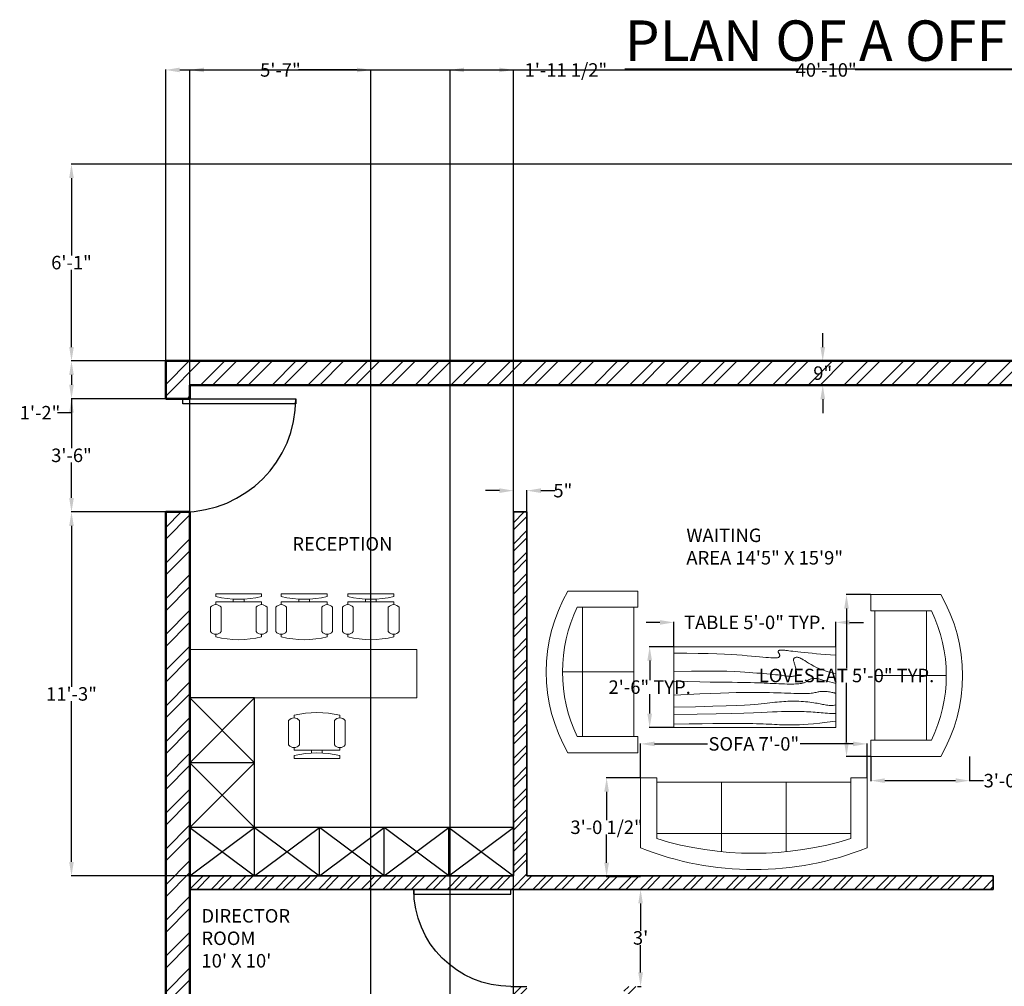
# Model space of a CAD drawing. Units: inches. Extents: x -355 to 263, y -871 to -163.
# Tile 5 of 6: x -355 to 10, y -521 to -163. Entities that reach past the tile are written whole.
import ezdxf

# ---------------------------------------------------------------- set-up
doc = ezdxf.new("R2010")
doc.units = ezdxf.units.IN
doc.header["$MEASUREMENT"] = 0
doc.layers.get('Defpoints').update_dxf_attribs({"color": 50})
for name, color, linetype, lineweight in [('A-ANNO-DIMS', 2, 'Continuous', 18), ('A-ANNO-TEXT', 7, 'Continuous', 25), ('A-AREA-IDEN', 7, 'Continuous', 18), ('A-FLOR-CASE', 9, 'Continuous', 25), ('A-WALL-PATT', 252, 'Continuous', 13)]:
    doc.layers.add(name, color=color, linetype=linetype, lineweight=lineweight)
for name, color, linetype, lineweight, plot in [('CHAIR', 8, 'Continuous', 18, False), ('DOOR', 4, 'Continuous', 25, False), ('IWAL', 7, 'Continuous', 35, False), ('OWALL', 7, 'Continuous', 50, False), ('SOFA', 8, 'Continuous', 18, False), ('TABLE', 8, 'Continuous', 18, False)]:
    doc.layers.add(name, color=color, linetype=linetype, lineweight=lineweight, plot=plot)
doc.styles.get("Standard").update_dxf_attribs({"font": 'arial.ttf'})
doc.dimstyles.get("Standard").update_dxf_attribs({"dimtxt": 5, "dimasz": 5.18, "dimexe": 0.18, "dimexo": 0.0625, "dimgap": 0.09, "dimtad": 0, "dimtih": 1, "dimtoh": 1, "dimdec": 0, "dimzin": 0, "dimdsep": 46, "dimlunit": 3, "dimtxsty": 'Standard', "dimcen": 0.09, "dimadec": 0, "dimazin": 0, "dimtfac": 1, "dimtdec": 0, "dimtofl": 0, "dimtmove": 0, "dimatfit": 3, "dimfxl": 1, "dimtolj": 1, "dimtzin": 0, "dimarcsym": 0})

# ---------------------------------------------------------------- blocks, each defined once
blk = doc.blocks.new('*U7')
for p, q in [((0, 0), (0, -6)), ((36, 0), (36, -6))]:
    blk.add_line(p, q)
blk.add_lwpolyline([(0, 0), (0, 36), (1.75, 36), (1.75, 0)], close=True)
blk.add_arc((0, 0), 36, 0, 90)
blk = doc.blocks.new('*U5')
for p, q in [((0, 0), (0, -6)), ((40, 0), (40, -6))]:
    blk.add_line(p, q)
blk.add_lwpolyline([(0, 0), (0, 40), (1.75, 40), (1.75, 0)], close=True)
blk.add_arc((0, 0), 40, 0, 90)
blk = doc.blocks.new('Chair - Desk')
for p, q in [((-8.5, 0), (-8.5, -1)), ((-8.5, 0), (8.5, 0)), ((8.5, 0), (8.5, -1)), ((-8.5, -3), (-8.5, -4)), ((-8.5, -3), (8.5, -3)), ((-2, -3), (-2, -1.9355)), ((2, -1.9576), (2, -3)), ((8.5, -3), (8.5, -4)), ((-10.5, -5), (-10.5, -14)), ((-6.5, -14), (-6.5, -5)), ((6.5, -5), (6.5, -14)), ((10.5, -14), (10.5, -5)), ((-8.5, -15), (-8.5, -16)), ((8.5, -15), (8.5, -16))]:
    blk.add_line(p, q)
for centre, radius, start, end in [((0, 34.625), 36.625, 256.5803, 283.4197), ((-8.5, -6.5), 2.5, 36.8699, 143.1301), ((8.5, -6.5), 2.5, 36.8699, 143.1301), ((-8.5, -12.5), 2.5, 216.8699, 323.1301), ((8.5, -12.5), 2.5, 216.8699, 323.1301), ((0, 19.625), 36.625, 256.5803, 283.4197)]:
    blk.add_arc(centre, radius, start, end)
blk = doc.blocks.new('Sofa - Roundback 7 ft.')
for p, q in [((-12.00002, -32.4421), (-12.00003, -6.5971)), ((11.99997, -32.4421), (11.99998, -6.5971)), ((-36.000027, -34), (-36.000027, -11.4696)), ((-35.999844, -13.3819), (35.9998, -13.3819)), ((35.99998, -34), (35.99998, -11.4696)), ((-36.000027, -32.4421), (35.99998, -32.4421))]:
    blk.add_line(p, q)
for points in [[(-36.000027, -34), (-42.000027, -34), (-42.000027, -8)], [(41.99998, -8), (41.99998, -34), (35.99998, -34)]]:
    blk.add_lwpolyline(points)
for centre, radius, start, end in [((0, -114.25), 114.25, 68.43141, 111.5686), ((-0.00001, -127.1968), 121.1968, 72.72033, 107.2797)]:
    blk.add_arc(centre, radius, start, end)
blk = doc.blocks.new('Sofa - Roundback Loveseat 5 ft.')
for p, q in [((0, -32.44198), (0, -5.99998)), ((-24, -33.99998), (-24, -11.46958)), ((-23.9998, -13.38178), (23.99986, -13.38178)), ((24.00004, -33.99998), (24.00004, -11.46958)), ((-24, -32.44198), (24.00004, -32.44198))]:
    blk.add_line(p, q)
for points in [[(-24, -33.99998), (-30, -33.99998), (-30, -7.99998)], [(30.00004, -7.99998), (30.00004, -33.99998), (24.00004, -33.99998)]]:
    blk.add_lwpolyline(points)
for centre, radius, start, end in [((0, -60.24998), 60.24998, 60.13715, 119.8628), ((0, -61.38438), 55.38444, 64.32083, 115.6792)]:
    blk.add_arc(centre, radius, start, end)
blk = doc.blocks.new('*D43')
at = {"layer": 'A-ANNO-DIMS', "color": 0, "lineweight": -2, "transparency": 16777216}
for p, q in [((-177.5, -337.37), (-182.68, -337.37)), ((-172.32, -345.22), (-172.32, -337.19)), ((-167.32, -345.22), (-167.32, -337.19)), ((-162.14, -337.37), (-156.96, -337.37))]:
    blk.add_line(p, q, dxfattribs=at)
at = {"layer": 'A-ANNO-DIMS', "color": 0, "lineweight": -3, "transparency": 16777216}
for points in [[(-177.5, -336.51), (-177.5, -338.24), (-172.32, -337.37)], [(-162.14, -336.51), (-162.14, -338.24), (-167.32, -337.37)]]:
    blk.add_solid(points, dxfattribs=at)
at = {"layer": 'Defpoints', "color": 0, "lineweight": -3, "transparency": 16777216}
for p in [(-167.32, -337.37), (-172.32, -345.28), (-167.32, -345.28)]:
    blk.add_point(p, dxfattribs=at)
at = {"layer": 'A-ANNO-DIMS', "color": 0, "transparency": 16777216, "insert": (-154, -337.37), "char_height": 5, "attachment_point": 5}
blk.add_mtext('\\A1;5"', dxfattribs=at)
blk = doc.blocks.new('*D44')
at = {"layer": 'A-ANNO-DIMS', "color": 0, "lineweight": -2, "transparency": 16777216}
for p, q in [((-57.59, -284.1), (-57.59, -278.92)), ((-80.81, -289.28), (-57.41, -289.28)), ((-80.81, -298.28), (-57.41, -298.28)), ((-57.59, -303.46), (-57.59, -308.64))]:
    blk.add_line(p, q, dxfattribs=at)
at = {"layer": 'A-ANNO-DIMS', "color": 0, "lineweight": -3, "transparency": 16777216}
for points in [[(-58.45, -284.1), (-56.72, -284.1), (-57.59, -289.28)], [(-58.45, -303.46), (-56.72, -303.46), (-57.59, -298.28)]]:
    blk.add_solid(points, dxfattribs=at)
at = {"layer": 'Defpoints', "color": 0, "lineweight": -3, "transparency": 16777216}
for p in [(-80.87, -289.28), (-80.87, -298.28), (-57.59, -298.28)]:
    blk.add_point(p, dxfattribs=at)
at = {"layer": 'A-ANNO-DIMS', "color": 0, "transparency": 16777216, "insert": (-57.59, -293.78), "char_height": 5, "attachment_point": 5}
blk.add_mtext('\\A1;9"', dxfattribs=at)
blk = doc.blocks.new('*D51')
at = {"layer": 'A-ANNO-DIMS', "color": 0, "lineweight": -2, "transparency": 16777216}
for p, q in [((-126.26, -485.28), (-124.98, -485.28)), ((-125.16, -490.46), (-125.16, -500.64)), ((-125.16, -516.1), (-125.16, -505.92)), ((-126.26, -521.28), (-124.98, -521.28))]:
    blk.add_line(p, q, dxfattribs=at)
at = {"layer": 'A-ANNO-DIMS', "color": 0, "lineweight": -3, "transparency": 16777216}
for points in [[(-126.02, -490.46), (-124.3, -490.46), (-125.16, -485.28)], [(-126.02, -516.1), (-124.3, -516.1), (-125.16, -521.28)]]:
    blk.add_solid(points, dxfattribs=at)
at = {"layer": 'Defpoints', "color": 0, "lineweight": -3, "transparency": 16777216}
for p in [(-126.32, -485.28), (-125.16, -485.28), (-126.32, -521.28)]:
    blk.add_point(p, dxfattribs=at)
at = {"layer": 'A-ANNO-DIMS', "color": 0, "transparency": 16777216, "insert": (-125.16, -503.28), "char_height": 5, "attachment_point": 5}
blk.add_mtext("\\A1;3'", dxfattribs=at)
blk = doc.blocks.new('Table - Rectangular Woodgrain 60 x 30 in.')
for p, q in [((0, 0), (0, -30)), ((60, 0), (0, 0)), ((60, -30), (60, 0)), ((0, -30), (60, -30))]:
    blk.add_line(p, q)
for points in [[(0, -2.4), (4.8155, -2.418), (9.0302, -2.4688), (12.709, -2.5477), (15.9167, -2.65), (18.7181, -2.7711), (21.1781, -2.9063), (23.3616, -3.0508), (25.3333, -3.2), (27.1477, -3.3495), (28.8172, -3.4958), (30.3437, -3.636), (31.7291, -3.7667), (32.9756, -3.8849), (34.0849, -3.9875), (35.059, -4.0714), (35.9, -4.1334), (36.6114, -4.1711), (37.2041, -4.1854), (37.6906, -4.1779), (38.0833, -4.15), (38.3948, -4.1034), (38.6375, -4.0396), (38.8239, -3.9602), (38.9666, -3.8667), (39.0764, -3.7608), (39.1573, -3.6448), (39.2116, -3.521), (39.2416, -3.3917), (39.2498, -3.2593), (39.2385, -3.1261), (39.21, -2.9944), (39.1666, -2.8667), (39.111, -2.7447), (39.0468, -2.6281), (38.978, -2.5163), (38.9083, -2.4083), (38.8418, -2.3035), (38.7823, -2.201), (38.7337, -2.1001), (38.7, -2), (38.6844, -1.9003), (38.6875, -1.8021), (38.7094, -1.707), (38.75, -1.6167), (38.8094, -1.5326), (38.8875, -1.4563), (38.9844, -1.3893), (39.1, -1.3333), (39.2351, -1.2896), (39.3937, -1.2583), (39.5804, -1.2396), (39.8, -1.2333), (40.057, -1.2396), (40.3562, -1.2583), (40.7023, -1.2896), (41.1, -1.3333), (41.5547, -1.3895), (42.0755, -1.4573), (42.6721, -1.5361), (43.3542, -1.625), (44.1316, -1.7233), (45.014, -1.8302), (46.0114, -1.9449), (47.1333, -2.0667), (48.3862, -2.1947), (49.7625, -2.3281), (51.2513, -2.4663), (52.8416, -2.6083), (54.5226, -2.7535), (56.2833, -2.9011), (58.1127, -3.0501), (60, -3.2)], [(0, -9.2), (6.5759, -9.0858), (11.9385, -9.0365), (16.2527, -9.0418), (19.6833, -9.0917), (22.3952, -9.1759), (24.5531, -9.2844), (26.322, -9.4069), (27.8666, -9.5333), (29.3241, -9.6553), (30.7203, -9.7719), (32.0532, -9.8837), (33.3208, -9.9917), (34.5213, -10.0965), (35.6526, -10.199), (36.7128, -10.2999), (37.7, -10.4), (38.6129, -10.4996), (39.4531, -10.5969), (40.223, -10.6895), (40.925, -10.775), (41.5613, -10.8512), (42.1344, -10.9156), (42.6465, -10.966), (43.1, -11), (43.4976, -11.0158), (43.8437, -11.0136), (44.143, -10.9942), (44.4, -10.9583), (44.6195, -10.9069), (44.8062, -10.8406), (44.9648, -10.7603), (45.1, -10.6667), (45.2155, -10.5598), (45.3114, -10.4365), (45.3871, -10.2929), (45.4416, -10.125), (45.4743, -9.929), (45.4844, -9.7011), (45.4709, -9.4371), (45.4333, -9.1333), (45.3716, -8.7883), (45.2896, -8.4104), (45.1919, -8.0107), (45.0833, -7.6), (44.9685, -7.1893), (44.8521, -6.7896), (44.7388, -6.4117), (44.6333, -6.0667), (44.54, -5.7628), (44.4614, -5.4979), (44.4001, -5.2675), (44.3583, -5.0667), (44.3384, -4.8909), (44.3427, -4.7354), (44.3736, -4.5956), (44.4333, -4.4667), (44.5236, -4.3453), (44.6427, -4.2333), (44.7884, -4.1339), (44.9583, -4.05), (45.1501, -3.9849), (45.3614, -3.9417), (45.59, -3.9234), (45.8333, -3.9333), (46.0915, -3.9749), (46.3734, -4.0531), (46.6906, -4.1736), (47.0542, -4.3417), (47.4756, -4.5629), (47.9661, -4.8427), (48.5372, -5.1866), (49.2, -5.6), (49.9676, -6.0844), (50.8594, -6.625), (51.8965, -7.2031), (53.1, -7.8), (54.491, -8.3969), (56.0906, -8.975), (57.9199, -9.5156), (60, -10)], [(0, -12.8), (5.1847, -12.9322), (9.6213, -13.0323), (13.3963, -13.1059), (16.5958, -13.1583), (19.3063, -13.1952), (21.614, -13.2219), (23.6054, -13.2439), (25.3666, -13.2667), (26.9728, -13.2947), (28.4531, -13.3281), (29.8256, -13.3663), (31.1083, -13.4083), (32.3191, -13.4535), (33.476, -13.501), (34.597, -13.5501), (35.7, -13.6), (36.7984, -13.6497), (37.8875, -13.6979), (38.9578, -13.743), (40, -13.7833), (41.0047, -13.8174), (41.9625, -13.8438), (42.864, -13.8607), (43.7, -13.8667), (44.4631, -13.8604), (45.1552, -13.8417), (45.7801, -13.8104), (46.3416, -13.7667), (46.8439, -13.7104), (47.2906, -13.6417), (47.6858, -13.5604), (48.0333, -13.4667), (48.3375, -13.3608), (48.6042, -13.2448), (48.8396, -13.121), (49.05, -12.9917), (49.2417, -12.8593), (49.4208, -12.7261), (49.5937, -12.5944), (49.7667, -12.4667), (49.9452, -12.3451), (50.1323, -12.2313), (50.3303, -12.1268), (50.5416, -12.0333), (50.7686, -11.9524), (51.0135, -11.8854), (51.2788, -11.8341), (51.5666, -11.8), (51.8785, -11.7843), (52.2116, -11.7865), (52.562, -11.8059), (52.926, -11.8417), (53.2998, -11.8931), (53.6795, -11.9594), (54.0614, -12.0397), (54.4416, -12.1333), (54.8223, -12.2401), (55.2293, -12.3625), (55.6942, -12.5037), (56.2489, -12.6667), (56.9251, -12.8547), (57.7545, -13.0708), (58.7689, -13.3182), (60, -13.6)], [(0, -18), (5.124, -17.7273), (9.6609, -17.5057), (13.6705, -17.3303), (17.2125, -17.1958), (20.3467, -17.0973), (23.1328, -17.0297), (25.6307, -16.9878), (27.9, -16.9667), (29.9928, -16.9617), (31.9302, -16.9703), (33.7254, -16.9907), (35.3917, -17.0208), (36.9423, -17.0588), (38.3906, -17.1026), (39.7499, -17.1503), (41.0333, -17.2), (42.2519, -17.2496), (43.4073, -17.2969), (44.4986, -17.3395), (45.525, -17.375), (46.4858, -17.4012), (47.3802, -17.4156), (48.2074, -17.416), (48.9667, -17.4), (49.6583, -17.3662), (50.2872, -17.3167), (50.8595, -17.2547), (51.3812, -17.1833), (51.8584, -17.1057), (52.2971, -17.025), (52.7034, -16.9443), (53.0833, -16.8667), (53.443, -16.7951), (53.789, -16.7313), (54.128, -16.6768), (54.4666, -16.6334), (54.8115, -16.6024), (55.1693, -16.5854), (55.5465, -16.5841), (55.95, -16.6), (56.3828, -16.6337), (56.8346, -16.6823), (57.2915, -16.7418), (57.7396, -16.8084), (58.165, -16.878), (58.5539, -16.9469), (58.8924, -17.0111), (59.1666, -17.0667), (59.3679, -17.1107), (59.5078, -17.1438), (59.6032, -17.1675), (59.6708, -17.1833), (59.7275, -17.193), (59.7901, -17.1979), (59.8753, -17.1998), (60, -17.2)], [(0, -22.4), (8.0098, -22.2501), (14.4094, -22.1011), (19.4168, -21.9535), (23.25, -21.8083), (26.1269, -21.6663), (28.2656, -21.5281), (29.884, -21.3947), (31.2, -21.2667), (32.3967, -21.1448), (33.5172, -21.0292), (34.5697, -20.9198), (35.5625, -20.8167), (36.5037, -20.7198), (37.4015, -20.6292), (38.2642, -20.5448), (39.1, -20.4667), (39.9164, -20.3951), (40.7187, -20.3313), (41.5117, -20.2768), (42.3, -20.2333), (43.0883, -20.2024), (43.8812, -20.1854), (44.6836, -20.1841), (45.5, -20.2), (46.3328, -20.234), (47.1747, -20.2844), (48.0163, -20.3488), (48.8479, -20.425), (49.66, -20.5106), (50.4429, -20.6031), (51.1872, -20.7004), (51.8833, -20.8), (52.5246, -20.8999), (53.1166, -20.9995), (53.6681, -21.0983), (54.1875, -21.1958), (54.6834, -21.2919), (55.1646, -21.3859), (55.6394, -21.4777), (56.1167, -21.5667), (56.6028, -21.6515), (57.0961, -21.7266), (57.5929, -21.7852), (58.0896, -21.8208), (58.5823, -21.8268), (59.0674, -21.7964), (59.5412, -21.723), (60, -21.6)], [(0, -25.2), (8.6355, -25.0504), (15.7026, -24.9031), (21.4049, -24.7606), (25.9458, -24.625), (29.529, -24.4988), (32.3578, -24.3844), (34.6359, -24.284), (36.5667, -24.2), (38.3213, -24.1341), (39.9417, -24.0854), (41.437, -24.0523), (42.8167, -24.0333), (44.0901, -24.0268), (45.2667, -24.0313), (46.3557, -24.0451), (47.3667, -24.0667), (48.309, -24.0947), (49.1928, -24.1287), (50.0284, -24.168), (50.826, -24.2125), (51.5959, -24.2617), (52.3483, -24.3151), (53.0935, -24.3725), (53.8417, -24.4334), (54.6009, -24.497), (55.3699, -24.561), (56.1454, -24.6226), (56.9239, -24.6792), (57.7021, -24.7279), (58.4764, -24.7662), (59.2435, -24.7911), (60, -24.8)], [(0, -28.8), (5.6867, -28.6681), (10.45, -28.5698), (14.407, -28.5012), (17.675, -28.4584), (20.3711, -28.4374), (22.6125, -28.4344), (24.5164, -28.4455), (26.2, -28.4667), (27.762, -28.4947), (29.2276, -28.5281), (30.6033, -28.5663), (31.8958, -28.6084), (33.1118, -28.6535), (34.2578, -28.7011), (35.3405, -28.7501), (36.3666, -28.8), (37.3443, -28.8497), (38.288, -28.8974), (39.2137, -28.9412), (40.1375, -28.9792), (41.0753, -29.0093), (42.0432, -29.0297), (43.0572, -29.0384), (44.1333, -29.0333), (45.2936, -29.0114), (46.5843, -28.9641), (48.0579, -28.8816), (49.7666, -28.7542), (51.7629, -28.5721), (54.0989, -28.3255), (56.8272, -28.0048), (60, -27.6)]]:
    blk.add_lwpolyline(points)
blk = doc.blocks.new('*D67')
at = {"layer": 'A-ANNO-DIMS', "color": 0, "lineweight": -2, "transparency": 16777216}
for p, q in [((-117.97, -386.25), (-123.15, -386.25)), ((-112.79, -395.19), (-112.79, -386.07)), ((-52.79, -395.19), (-52.79, -386.07)), ((-47.61, -386.25), (-42.43, -386.25))]:
    blk.add_line(p, q, dxfattribs=at)
at = {"layer": 'A-ANNO-DIMS', "color": 0, "lineweight": -3, "transparency": 16777216}
for points in [[(-117.97, -385.39), (-117.97, -387.11), (-112.79, -386.25)], [(-47.61, -385.39), (-47.61, -387.11), (-52.79, -386.25)]]:
    blk.add_solid(points, dxfattribs=at)
at = {"layer": 'Defpoints', "color": 0, "lineweight": -3, "transparency": 16777216}
for p in [(-52.79, -386.25), (-112.79, -395.25), (-52.79, -395.25)]:
    blk.add_point(p, dxfattribs=at)
at = {"layer": 'A-ANNO-DIMS', "color": 0, "transparency": 16777216, "insert": (-82.79, -386.25), "char_height": 5, "attachment_point": 5}
blk.add_mtext('\\A1;TABLE 5\'-0" TYP.', dxfattribs=at)
blk = doc.blocks.new('*D68')
at = {"layer": 'A-ANNO-DIMS', "color": 0, "lineweight": -2, "transparency": 16777216}
for p, q in [((-112.85, -395.25), (-121.97, -395.25)), ((-121.79, -400.43), (-121.79, -407.61)), ((-121.79, -420.07), (-121.79, -412.89)), ((-112.85, -425.25), (-121.97, -425.25))]:
    blk.add_line(p, q, dxfattribs=at)
at = {"layer": 'A-ANNO-DIMS', "color": 0, "lineweight": -3, "transparency": 16777216}
for points in [[(-122.66, -400.43), (-120.93, -400.43), (-121.79, -395.25)], [(-122.66, -420.07), (-120.93, -420.07), (-121.79, -425.25)]]:
    blk.add_solid(points, dxfattribs=at)
at = {"layer": 'Defpoints', "color": 0, "lineweight": -3, "transparency": 16777216}
for p in [(-121.79, -395.25), (-112.79, -395.25), (-112.79, -425.25)]:
    blk.add_point(p, dxfattribs=at)
at = {"layer": 'A-ANNO-DIMS', "color": 0, "transparency": 16777216, "insert": (-121.79, -410.25), "char_height": 5, "attachment_point": 5}
blk.add_mtext('\\A1;2\'-6" TYP.', dxfattribs=at)
blk = doc.blocks.new('*D69')
at = {"layer": 'A-ANNO-DIMS', "color": 0, "lineweight": -2, "transparency": 16777216}
for p, q in [((-39.83, -375.94), (-48.95, -375.94)), ((-48.77, -381.12), (-48.77, -403.26)), ((-48.77, -430.76), (-48.77, -408.61)), ((-39.83, -435.94), (-48.95, -435.94))]:
    blk.add_line(p, q, dxfattribs=at)
at = {"layer": 'A-ANNO-DIMS', "color": 0, "lineweight": -3, "transparency": 16777216}
for points in [[(-49.63, -381.12), (-47.91, -381.12), (-48.77, -375.94)], [(-49.63, -430.76), (-47.91, -430.76), (-48.77, -435.94)]]:
    blk.add_solid(points, dxfattribs=at)
at = {"layer": 'Defpoints', "color": 0, "lineweight": -3, "transparency": 16777216}
for p in [(-39.77, -375.94), (-48.77, -435.94), (-39.77, -435.94)]:
    blk.add_point(p, dxfattribs=at)
at = {"layer": 'A-ANNO-DIMS', "color": 0, "transparency": 16777216, "insert": (-48.77, -405.94), "char_height": 5, "attachment_point": 5}
blk.add_mtext('\\A1;LOVESEAT 5\'-0" TYP.', dxfattribs=at)
blk = doc.blocks.new('*D70')
at = {"layer": 'A-ANNO-DIMS', "color": 0, "lineweight": -2, "transparency": 16777216}
for p, q in [((-39.77, -436), (-39.77, -445.12)), ((-3.1, -436), (-3.1, -445.12)), ((-34.59, -444.94), (-8.28, -444.94)), ((-3.1, -444.94), (2.08, -444.94))]:
    blk.add_line(p, q, dxfattribs=at)
at = {"layer": 'A-ANNO-DIMS', "color": 0, "lineweight": -3, "transparency": 16777216}
for points in [[(-34.59, -444.07), (-34.59, -445.8), (-39.77, -444.94)], [(-8.28, -444.07), (-8.28, -445.8), (-3.1, -444.94)]]:
    blk.add_solid(points, dxfattribs=at)
at = {"layer": 'Defpoints', "color": 0, "lineweight": -3, "transparency": 16777216}
for p in [(-39.77, -435.94), (-3.1, -435.94), (-3.1, -444.94)]:
    blk.add_point(p, dxfattribs=at)
at = {"layer": 'A-ANNO-DIMS', "color": 0, "transparency": 16777216, "insert": (23.23, -444.94), "char_height": 5, "attachment_point": 5}
blk.add_mtext('\\A1;3\'-0 1/2" TYP.', dxfattribs=at)
blk = doc.blocks.new('*D73')
at = {"layer": 'A-ANNO-DIMS', "color": 0, "lineweight": -2, "transparency": 16777216}
for p, q in [((-125.16, -443.84), (-125.16, -431.12)), ((-119.98, -431.3), (-100.36, -431.3)), ((-46.34, -431.3), (-65.96, -431.3)), ((-41.16, -443.84), (-41.16, -431.12))]:
    blk.add_line(p, q, dxfattribs=at)
at = {"layer": 'A-ANNO-DIMS', "color": 0, "lineweight": -3, "transparency": 16777216}
for points in [[(-119.98, -430.44), (-119.98, -432.16), (-125.16, -431.3)], [(-46.34, -430.44), (-46.34, -432.16), (-41.16, -431.3)]]:
    blk.add_solid(points, dxfattribs=at)
at = {"layer": 'Defpoints', "color": 0, "lineweight": -3, "transparency": 16777216}
for p in [(-125.16, -431.3), (-125.16, -443.9), (-41.16, -443.9)]:
    blk.add_point(p, dxfattribs=at)
at = {"layer": 'A-ANNO-DIMS', "color": 0, "transparency": 16777216, "insert": (-83.16, -431.3), "char_height": 5, "attachment_point": 5}
blk.add_mtext('\\A1;SOFA 7\'-0"', dxfattribs=at)
blk = doc.blocks.new('*D74')
at = {"layer": 'A-ANNO-DIMS', "color": 0, "lineweight": -2, "transparency": 16777216}
for p, q in [((-125.22, -443.9), (-137.94, -443.9)), ((-137.76, -449.08), (-137.76, -459.56)), ((-137.76, -475.39), (-137.76, -464.91)), ((-125.22, -480.57), (-137.94, -480.57))]:
    blk.add_line(p, q, dxfattribs=at)
at = {"layer": 'A-ANNO-DIMS', "color": 0, "lineweight": -3, "transparency": 16777216}
for points in [[(-138.63, -449.08), (-136.9, -449.08), (-137.76, -443.9)], [(-138.63, -475.39), (-136.9, -475.39), (-137.76, -480.57)]]:
    blk.add_solid(points, dxfattribs=at)
at = {"layer": 'Defpoints', "color": 0, "lineweight": -3, "transparency": 16777216}
for p in [(-125.16, -443.9), (-137.76, -480.57), (-125.16, -480.57)]:
    blk.add_point(p, dxfattribs=at)
at = {"layer": 'A-ANNO-DIMS', "color": 0, "transparency": 16777216, "insert": (-137.76, -462.23), "char_height": 5, "attachment_point": 5}
blk.add_mtext('\\A1;3\'-0 1/2"', dxfattribs=at)
blk = doc.blocks.new('*D75')
at = {"layer": 'A-ANNO-DIMS', "color": 0, "lineweight": -2, "transparency": 16777216}
for p, q in [((-301.32, -289.22), (-301.32, -181.15)), ((-296.14, -181.33), (-67.04, -181.33)), ((183.5, -181.33), (-45.6, -181.33)), ((188.68, -216.22), (188.68, -181.15))]:
    blk.add_line(p, q, dxfattribs=at)
at = {"layer": 'A-ANNO-DIMS', "color": 0, "lineweight": -3, "transparency": 16777216}
for points in [[(-296.14, -180.47), (-296.14, -182.19), (-301.32, -181.33)], [(183.5, -180.47), (183.5, -182.19), (188.68, -181.33)]]:
    blk.add_solid(points, dxfattribs=at)
at = {"layer": 'Defpoints', "color": 0, "lineweight": -3, "transparency": 16777216}
for p in [(188.68, -181.33), (188.68, -216.28), (-301.32, -289.28)]:
    blk.add_point(p, dxfattribs=at)
at = {"layer": 'A-ANNO-DIMS', "color": 0, "transparency": 16777216, "insert": (-56.32, -181.33), "char_height": 5, "attachment_point": 5}
blk.add_mtext('\\A1;40\'-10"', dxfattribs=at)
blk = doc.blocks.new('*D77')
at = {"layer": 'A-ANNO-DIMS', "color": 0, "lineweight": -2, "transparency": 16777216}
for p, q in [((54.62, -216.28), (-336.45, -216.28)), ((-336.27, -221.46), (-336.27, -250.14)), ((-336.27, -284.1), (-336.27, -255.42)), ((54.62, -289.28), (-336.45, -289.28))]:
    blk.add_line(p, q, dxfattribs=at)
at = {"layer": 'A-ANNO-DIMS', "color": 0, "lineweight": -3, "transparency": 16777216}
for points in [[(-337.13, -221.46), (-335.41, -221.46), (-336.27, -216.28)], [(-337.13, -284.1), (-335.41, -284.1), (-336.27, -289.28)]]:
    blk.add_solid(points, dxfattribs=at)
at = {"layer": 'Defpoints', "color": 0, "lineweight": -3, "transparency": 16777216}
for p in [(-336.27, -216.28), (54.68, -216.28), (54.68, -289.28)]:
    blk.add_point(p, dxfattribs=at)
at = {"layer": 'A-ANNO-DIMS', "color": 0, "transparency": 16777216, "insert": (-336.27, -252.78), "char_height": 5, "attachment_point": 5}
blk.add_mtext('\\A1;6\'-1"', dxfattribs=at)
blk = doc.blocks.new('*D78')
at = {"layer": 'A-ANNO-DIMS', "color": 0, "lineweight": -2, "transparency": 16777216}
for p, q in [((-301.38, -303.28), (-336.45, -303.28)), ((-336.27, -308.46), (-336.27, -321.64)), ((-336.27, -340.1), (-336.27, -326.92)), ((-301.38, -345.28), (-336.45, -345.28))]:
    blk.add_line(p, q, dxfattribs=at)
at = {"layer": 'A-ANNO-DIMS', "color": 0, "lineweight": -3, "transparency": 16777216}
for points in [[(-337.13, -308.46), (-335.41, -308.46), (-336.27, -303.28)], [(-337.13, -340.1), (-335.41, -340.1), (-336.27, -345.28)]]:
    blk.add_solid(points, dxfattribs=at)
at = {"layer": 'Defpoints', "color": 0, "lineweight": -3, "transparency": 16777216}
for p in [(-301.32, -303.28), (-336.27, -345.28), (-301.32, -345.28)]:
    blk.add_point(p, dxfattribs=at)
at = {"layer": 'A-ANNO-DIMS', "color": 0, "transparency": 16777216, "insert": (-336.27, -324.28), "char_height": 5, "attachment_point": 5}
blk.add_mtext('\\A1;3\'-6"', dxfattribs=at)
blk = doc.blocks.new('*D81')
at = {"layer": 'A-ANNO-DIMS', "color": 0, "lineweight": -2, "transparency": 16777216}
for p, q in [((-301.38, -289.28), (-336.45, -289.28)), ((-336.27, -294.46), (-336.27, -298.1)), ((-301.38, -303.28), (-336.45, -303.28)), ((-336.27, -303.28), (-336.27, -308.46)), ((-336.27, -308.46), (-341.45, -308.46))]:
    blk.add_line(p, q, dxfattribs=at)
at = {"layer": 'A-ANNO-DIMS', "color": 0, "lineweight": -3, "transparency": 16777216}
for points in [[(-337.13, -294.46), (-335.41, -294.46), (-336.27, -289.28)], [(-337.13, -298.1), (-335.41, -298.1), (-336.27, -303.28)]]:
    blk.add_solid(points, dxfattribs=at)
at = {"layer": 'Defpoints', "color": 0, "lineweight": -3, "transparency": 16777216}
for p in [(-301.32, -289.28), (-336.27, -303.28), (-301.32, -303.28)]:
    blk.add_point(p, dxfattribs=at)
at = {"layer": 'A-ANNO-DIMS', "color": 0, "transparency": 16777216, "insert": (-347.95, -308.46), "char_height": 5, "attachment_point": 5}
blk.add_mtext('\\A1;1\'-2"', dxfattribs=at)
blk = doc.blocks.new('*D84')
at = {"layer": 'A-ANNO-DIMS', "color": 0, "lineweight": -2, "transparency": 16777216}
for p, q in [((-195.8, -605.22), (-195.8, -181.15)), ((-190.62, -181.33), (-177.5, -181.33)), ((-172.32, -605.22), (-172.32, -181.15)), ((-172.32, -181.33), (-167.14, -181.33))]:
    blk.add_line(p, q, dxfattribs=at)
at = {"layer": 'A-ANNO-DIMS', "color": 0, "lineweight": -3, "transparency": 16777216}
for points in [[(-190.62, -180.47), (-190.62, -182.19), (-195.8, -181.33)], [(-177.5, -180.47), (-177.5, -182.19), (-172.32, -181.33)]]:
    blk.add_solid(points, dxfattribs=at)
at = {"layer": 'Defpoints', "color": 0, "lineweight": -3, "transparency": 16777216}
for p in [(-172.32, -181.33), (-195.8, -605.28), (-172.32, -605.28)]:
    blk.add_point(p, dxfattribs=at)
at = {"layer": 'A-ANNO-DIMS', "color": 0, "transparency": 16777216, "insert": (-152.87, -181.33), "char_height": 5, "attachment_point": 5}
blk.add_mtext('\\A1;1\'-11 1/2"', dxfattribs=at)
blk = doc.blocks.new('*D85')
at = {"layer": 'A-ANNO-DIMS', "color": 0, "lineweight": -2, "transparency": 16777216}
for p, q in [((-292.32, -610.22), (-292.32, -181.15)), ((-287.14, -181.33), (-265.5, -181.33)), ((-230.39, -181.33), (-252.03, -181.33)), ((-225.21, -620.24), (-225.21, -181.15))]:
    blk.add_line(p, q, dxfattribs=at)
at = {"layer": 'A-ANNO-DIMS', "color": 0, "lineweight": -3, "transparency": 16777216}
for points in [[(-287.14, -180.47), (-287.14, -182.19), (-292.32, -181.33)], [(-230.39, -180.47), (-230.39, -182.19), (-225.21, -181.33)]]:
    blk.add_solid(points, dxfattribs=at)
at = {"layer": 'Defpoints', "color": 0, "lineweight": -3, "transparency": 16777216}
for p in [(-225.21, -181.33), (-292.32, -610.28), (-225.21, -620.3)]:
    blk.add_point(p, dxfattribs=at)
at = {"layer": 'A-ANNO-DIMS', "color": 0, "transparency": 16777216, "insert": (-258.76, -181.33), "char_height": 5, "attachment_point": 5}
blk.add_mtext('\\A1;5\'-7"', dxfattribs=at)
blk = doc.blocks.new('*D95')
at = {"layer": 'A-ANNO-DIMS', "color": 0, "lineweight": -2, "transparency": 16777216}
for p, q in [((-301.38, -345.28), (-336.45, -345.28)), ((-336.27, -350.46), (-336.27, -410.14)), ((-336.27, -475.1), (-336.27, -415.42)), ((-292.38, -480.28), (-336.45, -480.28))]:
    blk.add_line(p, q, dxfattribs=at)
at = {"layer": 'A-ANNO-DIMS', "color": 0, "lineweight": -3, "transparency": 16777216}
for points in [[(-337.13, -350.46), (-335.41, -350.46), (-336.27, -345.28)], [(-337.13, -475.1), (-335.41, -475.1), (-336.27, -480.28)]]:
    blk.add_solid(points, dxfattribs=at)
at = {"layer": 'Defpoints', "color": 0, "lineweight": -3, "transparency": 16777216}
for p in [(-301.32, -345.28), (-336.27, -480.28), (-292.32, -480.28)]:
    blk.add_point(p, dxfattribs=at)
at = {"layer": 'A-ANNO-DIMS', "color": 0, "transparency": 16777216, "insert": (-336.27, -412.78), "char_height": 5, "attachment_point": 5}
blk.add_mtext('\\A1;11\'-3"', dxfattribs=at)

msp = doc.modelspace()

# ---------------------------------------------------------------- hatches: boundary and pattern name
at = {"layer": 'A-WALL-PATT'}
h = msp.add_hatch(dxfattribs=at)
h.set_pattern_fill('ANSI32', color=256, scale=25)
h.set_pattern_definition([(45, (-301.32, -828.28), (-6.62913, 6.62913), []), (45, (-296.9, -828.28), (-6.62913, 6.62913), [])])
h.paths.add_polyline_path([(54.68, -289.28), (-301.32, -289.28), (-301.32, -303.28), (-295.02, -303.28), (-292.32, -303.28), (-292.32, -298.28), (54.68, -298.28)])
h.paths.add_polyline_path([(188.68, -216.28), (54.68, -216.28), (54.68, -225.28), (179.68, -225.28), (179.68, -345.28), (179.68, -485.16), (184.18, -485.16), (188.68, -485.16)])
h.paths.add_polyline_path([(188.68, -521.16), (184.18, -521.16), (179.68, -521.16), (179.68, -540.28), (188.68, -540.28)])
h.paths.add_polyline_path([(164.68, -540.28), (155.68, -540.28), (155.68, -552.97), (160.18, -552.97), (164.68, -552.97)])
h.paths.add_polyline_path([(164.68, -588.97), (160.18, -588.97), (155.68, -588.97), (155.68, -620.04), (160.18, -620.04), (164.68, -620.04)])
h.paths.add_polyline_path([(164.68, -656.04), (160.18, -656.04), (155.68, -656.04), (155.68, -682.06), (160.18, -682.06), (164.68, -682.06)])
h.paths.add_polyline_path([(164.68, -718.06), (160.18, -718.06), (155.68, -718.06), (155.68, -730.28), (164.68, -730.28)])
h.paths.add_polyline_path([(188.68, -730.28), (179.68, -730.28), (179.68, -819.28), (73.9, -819.28), (73.9, -823.78), (73.9, -828.28), (188.68, -828.28)])
h.paths.add_polyline_path([(25.9, -819.28), (-41.45, -819.28), (-41.45, -823.78), (-41.45, -828.28), (25.9, -828.28), (25.9, -823.78)])
h.paths.add_polyline_path([(-113.45, -819.28), (-292.32, -819.28), (-292.32, -796.14), (-296.82, -796.14), (-301.32, -796.14), (-301.32, -828.28), (-113.45, -828.28), (-113.45, -823.78)])
h.paths.add_polyline_path([(-292.32, -480.28), (-292.32, -345.28), (-301.32, -345.28), (-301.32, -620.18), (-296.82, -620.18), (-292.32, -620.18)])
h.paths.add_polyline_path([(-292.32, -656.18), (-296.82, -656.18), (-301.32, -656.18), (-301.32, -700.14), (-296.82, -700.14), (-292.32, -700.14)])
h = msp.add_hatch(dxfattribs=at)
h.set_pattern_fill('ANSI32', color=256, scale=15)
h.set_pattern_definition([(45, (-292.3197, -819.28), (-3.977476, 3.977476), []), (45, (-289.668, -819.28), (-3.977476, 3.977476), [])])
h.paths.add_polyline_path([(59.68, -280.18), (57.18, -280.18), (54.68, -280.18), (54.68, -289.28), (54.68, -298.28), (54.68, -303.28), (59.68, -303.28)])
h.paths.add_polyline_path([(59.68, -225.28), (54.68, -225.28), (54.68, -232.18), (57.18, -232.18), (59.68, -232.18)])
h.paths.add_polyline_path([(18.68, -641.28), (18.68, -521.28), (13.68, -521.28), (13.68, -641.28), (-7.32, -665.28), (-105.32, -665.28), (-126.32, -641.28), (-126.32, -521.28), (-131.32, -521.28), (-131.32, -641.28), (-105.32, -670.28), (-7.32, -670.28)])
h.paths.add_polyline_path([(-167.32, -521.28), (-172.32, -521.28), (-172.32, -538.25), (-169.82, -538.25), (-167.32, -538.25)])
h.paths.add_polyline_path([(-134.32, -670.28), (-167.32, -670.28), (-167.32, -610.28), (-167.32, -586.25), (-169.82, -586.25), (-172.32, -586.25), (-172.32, -670.28), (-292.32, -670.28), (-292.32, -675.28), (-139.32, -675.28), (-134.32, -675.28)])
h.paths.add_polyline_path([(-167.32, -345.28), (-172.32, -345.28), (-172.32, -462.28), (-172.32, -480.28), (-292.32, -480.28), (-292.32, -485.28), (-172.32, -485.28), (-167.32, -485.28), (5.68, -485.28), (5.68, -480.28), (-167.32, -480.28)])
h.paths.add_polyline_path([(179.68, -345.28), (30.68, -345.28), (30.68, -365.65), (33.18, -365.65), (35.68, -365.65), (35.68, -350.28), (179.68, -350.28)])
h.paths.add_polyline_path([(-134.32, -707.28), (-139.32, -707.28), (-139.32, -819.28), (-134.32, -819.28)])
h.paths.add_polyline_path([(-9.32, -707.28), (-102.32, -707.28), (-102.32, -712.28), (-14.32, -712.28), (-14.32, -819.28), (-9.32, -819.28)])
h.paths.add_polyline_path([(179.68, -730.28), (22.68, -730.28), (22.68, -735.28), (179.68, -735.28)])
h.paths.add_polyline_path([(179.68, -470.28), (30.68, -470.28), (30.68, -475.28), (54.68, -475.28), (54.68, -505.29), (59.18, -505.29, -0.00418), (59.68, -505.29), (59.68, -475.28), (179.68, -475.28)])
h.paths.add_polyline_path([(35.68, -413.65), (33.18, -413.65), (30.68, -413.65), (30.68, -440.29), (35.18, -440.29, -0.00418), (35.68, -440.29)])
h.paths.add_polyline_path([(179.68, -535.28), (54.68, -535.28), (54.68, -540.28), (54.68, -570.29), (59.18, -570.29, -0.00418), (59.68, -570.29), (59.68, -540.28), (179.68, -540.28)])
h.paths.add_polyline_path([(121.93, -531.51), (160.73, -531.51), (160.73, -512.85), (121.93, -512.85)], flags=9)
h.paths.add_polyline_path([(49.47, -376.48), (111.2, -376.48), (111.2, -357.82), (49.47, -357.82)], flags=9)

# ---------------------------------------------------------------- linework, layer by layer
at = {"layer": 'A-FLOR-CASE'}
for p, q in [((-268.32, -414.28), (-292.32, -414.28)), ((-292.32, -438.28), (-268.32, -414.28)), ((-268.32, -438.28), (-292.32, -414.28)), ((-268.32, -462.28), (-268.32, -414.28)), ((-268.32, -438.28), (-292.32, -438.28)), ((-292.32, -438.28), (-268.32, -462.28)), ((-268.32, -438.28), (-292.32, -462.28)), ((-172.32, -462.28), (-292.32, -462.28)), ((-292.32, -480.28), (-268.32, -462.28)), ((-292.32, -462.28), (-268.32, -480.28)), ((-268.32, -480.28), (-268.32, -462.28)), ((-268.32, -480.28), (-244.32, -462.28)), ((-268.32, -462.28), (-244.32, -480.28)), ((-244.32, -480.28), (-244.32, -462.28)), ((-244.32, -480.28), (-220.32, -462.28)), ((-220.32, -480.28), (-244.32, -462.28)), ((-220.32, -480.28), (-220.32, -462.28)), ((-220.32, -480.28), (-196.32, -462.28)), ((-196.32, -480.28), (-220.32, -462.28)), ((-196.32, -480.28), (-196.32, -462.28)), ((-196.32, -480.28), (-172.32, -462.28)), ((-196.32, -462.28), (-172.32, -480.28))]:
    msp.add_line(p, q, dxfattribs=at)
at = {"layer": 'IWAL'}
for p, q in [((-172.32, -345.28), (-167.32, -345.28)), ((-172.32, -462.28), (-172.32, -345.28)), ((-167.32, -480.28), (-167.32, -345.28)), ((-172.32, -480.28), (-172.32, -462.28)), ((-172.32, -480.28), (-292.32, -480.28)), ((5.68, -480.28), (-167.32, -480.28)), ((5.68, -485.28), (5.68, -480.28)), ((-172.32, -485.28), (-292.32, -485.28)), ((5.68, -485.28), (-172.32, -485.28))]:
    msp.add_line(p, q, dxfattribs=at)
at = {"layer": 'OWALL'}
for p, q in [((54.68, -289.28), (-301.32, -289.28)), ((-301.32, -303.28), (-301.32, -289.28)), ((54.68, -298.28), (-292.32, -298.28)), ((-292.32, -303.28), (-292.32, -298.28)), ((-292.32, -303.28), (-301.32, -303.28)), ((-301.32, -828.28), (-301.32, -345.28)), ((-292.32, -345.28), (-301.32, -345.28)), ((-292.32, -480.28), (-292.32, -345.28)), ((-292.32, -819.28), (-292.32, -480.28))]:
    msp.add_line(p, q, dxfattribs=at)
at = {"layer": 'TABLE'}
for p, q in [((-208.21, -396.28), (-292.32, -396.28)), ((-208.21, -414.28), (-208.21, -396.28)), ((-268.32, -414.28), (-208.21, -414.28))]:
    msp.add_line(p, q, dxfattribs=at)

# ---------------------------------------------------------------- block references
at = {"layer": 'CHAIR'}
for p in [(-274.24, -375.65), (-249.95, -375.65), (-225.25, -375.65)]:
    msp.add_blockref('Chair - Desk', p, dxfattribs=at)
at = {"layer": 'CHAIR', "rotation": 180}
msp.add_blockref('Chair - Desk', (-245.22, -436.67), dxfattribs=at)
at = {"layer": 'DOOR', "xscale": 1.05, "yscale": 1.05, "zscale": 1.05, "rotation": 270}
msp.add_blockref('*U5', (-295.02, -303.28), dxfattribs=at)
at = {"layer": 'DOOR', "xscale": -1, "rotation": 90}
msp.add_blockref('*U7', (-173.32, -485.28), dxfattribs=at)
at = {"layer": 'SOFA'}
for name, p, rotation in [('Sofa - Roundback Loveseat 5 ft.', (-160.15, -404.62), 90), ('Sofa - Roundback Loveseat 5 ft.', (-5.77, -405.94), 270), ('Sofa - Roundback 7 ft.', (-83.16, -477.9), 180)]:
    msp.add_blockref(name, p, dxfattribs=dict(at, rotation=rotation))
at = {"layer": 'TABLE'}
msp.add_blockref('Table - Rectangular Woodgrain 60 x 30 in.', (-112.79, -395.25), dxfattribs=at)

# ---------------------------------------------------------------- texts
at = {"layer": 'A-ANNO-TEXT', "insert": (-131.06, -162.96), "char_height": 15, "attachment_point": 1}
msp.add_mtext_dynamic_manual_height_columns('{\\fArial|b1|i0|c0|p34;\\LPLAN OF A OFFICE BUILDING}', width=417.8492, gutter_width=1, heights=[0], dxfattribs=at)
at = {"layer": 'A-AREA-IDEN', "char_height": 5, "attachment_point": 1}
for s, width, insert in [('{WAITING\\PAREA 14\'5" X 15\'9"}', 113.3298, (-108.17, -351.44)), ('{RECEPTION}', 31.7783, (-254.35, -354.62)), ("{DIRECTOR\\PROOM\\P10' X 10'}", 59.9561, (-288.05, -492.58))]:
    msp.add_mtext_dynamic_manual_height_columns(s, width=width, gutter_width=1, heights=[0], dxfattribs=dict(at, insert=insert))

# ---------------------------------------------------------------- dimensions: what is measured, and where the dimension line sits
at = {"layer": 'A-ANNO-DIMS'}
for base, p1, p2, override, picture, middle in [((-172.32, -181.33), (-195.8, -605.28), (-172.32, -605.28), {"dimdec": 1, "dimlfac": 1, "dimrnd": 0, "dimzin": 1, "dimdsep": 46, "dimlunit": 4, "dimfrac": 2}, '*D84', (-152.87, -181.33)), ((188.68, -181.33), (-301.32, -289.28), (188.68, -216.28), {"dimdec": 1, "dimlfac": 1, "dimrnd": 0, "dimzin": 1, "dimdsep": 46, "dimlunit": 4, "dimfrac": 2}, '*D75', (-56.32, -181.33)), ((-225.21, -181.33), (-292.32, -610.28), (-225.21, -620.3), {"dimdec": 1, "dimlfac": 1, "dimrnd": 0, "dimzin": 1, "dimdsep": 46, "dimlunit": 4, "dimfrac": 2}, '*D85', (-258.76, -181.33)), ((-167.32, -337.37), (-172.32, -345.28), (-167.32, -345.28), {"dimclrd": 0, "dimclre": 0, "dimclrt": 0}, '*D43', (-154, -337.37))]:
    dim = msp.add_linear_dim(base=base, p1=p1, p2=p2, dimstyle='Standard', override=override, dxfattribs=at)
    dim.commit()
    dim.dimension.update_dxf_attribs({"geometry": picture, "text_midpoint": middle})
for base, p1, p2, angle, override, picture, middle in [((-336.27, -216.28), (54.68, -289.28), (54.68, -216.28), 90, {"dimdec": 1, "dimlfac": 1, "dimrnd": 0, "dimzin": 1, "dimdsep": 46, "dimlunit": 4, "dimfrac": 2}, '*D77', (-336.27, -252.78)), ((-57.59, -298.28), (-80.87, -289.28), (-80.87, -298.28), 90, {"dimclrd": 0, "dimclre": 0, "dimclrt": 0}, '*D44', (-57.59, -293.78)), ((-336.27, -303.28), (-301.32, -289.28), (-301.32, -303.28), 90, {"dimdec": 1, "dimlfac": 1, "dimrnd": 0, "dimzin": 1, "dimdsep": 46, "dimlunit": 4, "dimfrac": 2}, '*D81', (-347.95, -308.46)), ((-336.27, -345.28), (-301.32, -303.28), (-301.32, -345.28), 90, {"dimdec": 1, "dimlfac": 1, "dimrnd": 0, "dimzin": 1, "dimdsep": 46, "dimlunit": 4, "dimfrac": 2}, '*D78', (-336.27, -324.28)), ((-336.27, -480.28), (-301.32, -345.28), (-292.32, -480.28), 90, {"dimdec": 1, "dimlfac": 1, "dimrnd": 0, "dimzin": 1, "dimdsep": 46, "dimlunit": 4, "dimfrac": 2}, '*D95', (-336.27, -412.78)), ((-137.76, -480.57), (-125.16, -443.9), (-125.16, -480.57), 270, {"dimdec": 1, "dimlfac": 1, "dimrnd": 0, "dimzin": 1, "dimdsep": 46, "dimlunit": 4, "dimfrac": 2}, '*D74', (-137.76, -462.23)), ((-125.16, -485.28), (-126.32, -521.28), (-126.32, -485.28), 90, {"dimclrd": 0, "dimclre": 0, "dimclrt": 0}, '*D51', (-125.16, -503.28))]:
    dim = msp.add_linear_dim(base=base, p1=p1, p2=p2, angle=angle, dimstyle='Standard', override=override, dxfattribs=at)
    dim.commit()
    dim.dimension.update_dxf_attribs({"geometry": picture, "text_midpoint": middle})
for base, p1, p2, text, picture, middle in [((-52.79, -386.25), (-112.79, -395.25), (-52.79, -395.25), 'TABLE <> TYP.', '*D67', (-82.79, -386.25)), ((-3.1, -444.94), (-39.77, -435.94), (-3.1, -435.94), '<> TYP.', '*D70', (23.23, -444.94))]:
    dim = msp.add_linear_dim(base=base, p1=p1, p2=p2, text=text, dimstyle='Standard', override={"dimdec": 1, "dimlfac": 1, "dimrnd": 0, "dimzin": 1, "dimdsep": 46, "dimlunit": 4, "dimfrac": 2}, dxfattribs=at)
    dim.commit()
    dim.dimension.update_dxf_attribs({"geometry": picture, "text_midpoint": middle})
for base, p1, p2, angle, text, picture, middle in [((-48.77, -435.94), (-39.77, -375.94), (-39.77, -435.94), 270, 'LOVESEAT <> TYP.', '*D69', (-48.77, -405.94)), ((-121.79, -395.25), (-112.79, -425.25), (-112.79, -395.25), 90, '<> TYP.', '*D68', (-121.79, -410.25)), ((-125.16, -431.3), (-41.16, -443.9), (-125.16, -443.9), 180, 'SOFA <>', '*D73', (-83.16, -431.3))]:
    dim = msp.add_linear_dim(base=base, p1=p1, p2=p2, angle=angle, text=text, dimstyle='Standard', override={"dimdec": 1, "dimlfac": 1, "dimrnd": 0, "dimzin": 1, "dimdsep": 46, "dimlunit": 4, "dimfrac": 2}, dxfattribs=at)
    dim.commit()
    dim.dimension.update_dxf_attribs({"geometry": picture, "text_midpoint": middle})

doc.saveas('drawing.dxf')
